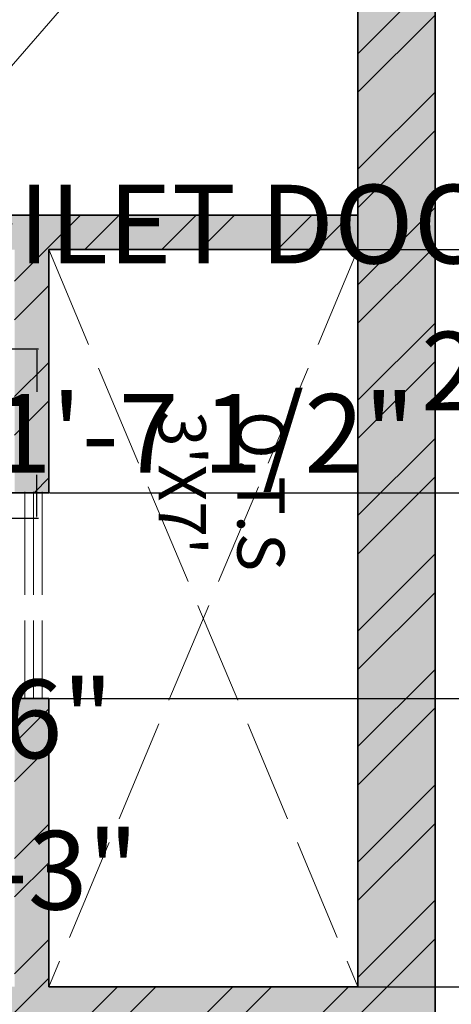
# Model space of a CAD drawing. Units: inches. Extents: x 1086 to 1540, y 3343 to 3848.
# Tile 5 of 8: x 1422 to 1473, y 3547 to 3661. Entities that reach past the tile are written whole.
import ezdxf

# ---------------------------------------------------------------- set-up
doc = ezdxf.new("R2010")
doc.units = ezdxf.units.IN
doc.linetypes.add('ACAD_ISO02W100', pattern=[15, 12, -3])
for name, color, linetype, lineweight in [('00 FURNITURE', 15, 'Continuous', 15), ('A-ANNO-DIMS', 2, 'Continuous', 13), ('A-AREA-IDEN', 7, 'Continuous', 18), ('A-FLOR-OPEN', 8, 'ACAD_ISO02W100', 13), ('A-GLAZ-VENT', 6, 'ACAD_ISO02W100', 13), ('A-WALL-PATT', 252, 'Continuous', 9), ('WALL', 7, 'Continuous', 35)]:
    doc.layers.add(name, color=color, linetype=linetype, lineweight=lineweight)
doc.styles.get("Standard").update_dxf_attribs({"font": 'arial.ttf'})
doc.dimstyles.get("Standard").update_dxf_attribs({"dimtxt": 9.18, "dimasz": 0.18, "dimexe": 0.18, "dimexo": 0.0625, "dimgap": 0.09, "dimtad": 0, "dimtih": 1, "dimtoh": 1, "dimdec": 1, "dimzin": 0, "dimdsep": 46, "dimlunit": 3, "dimtxsty": 'Standard', "dimcen": 0.09, "dimadec": 0, "dimazin": 0, "dimtfac": 1, "dimtdec": 1, "dimtofl": 0, "dimtmove": 0, "dimatfit": 3, "dimfxl": 1, "dimtolj": 1, "dimtzin": 0, "dimarcsym": 0})

# ---------------------------------------------------------------- blocks, each defined once
blk = doc.blocks.new('chair')
at = {"layer": '00 FURNITURE'}
for p, q in [((1375.85, 3529.75), (1402.12, 3529.75)), ((1373.66, 3525.37), (1373.66, 3527.56)), ((1404.31, 3527.56), (1404.31, 3496.9)), ((1371.47, 3525.37), (1397.74, 3525.37)), ((1395.55, 3525.37), (1395.55, 3499.09)), ((1369.28, 3501.28), (1369.28, 3523.18)), ((1399.93, 3523.18), (1399.93, 3501.28)), ((1397.74, 3499.09), (1371.47, 3499.09)), ((1373.66, 3496.9), (1373.66, 3499.09)), ((1402.12, 3494.71), (1375.85, 3494.71))]:
    blk.add_line(p, q, dxfattribs=at)
for centre, start, end in [((1375.85, 3527.56), 90, 180), ((1402.12, 3527.56), 0, 90), ((1371.47, 3523.18), 90, 180), ((1397.74, 3523.18), 0, 90), ((1371.47, 3501.28), 180, 270), ((1397.74, 3501.28), 270, 0), ((1375.85, 3496.9), 180, 270), ((1402.12, 3496.9), 270, 0)]:
    blk.add_arc(centre, 2.19, start, end, dxfattribs=at)
blk = doc.blocks.new('*D13')
at = {"layer": 'A-ANNO-DIMS', "color": 0, "lineweight": -2, "transparency": 16777216}
for p, q in [((1470.8, 3811.57), (1506.93, 3811.57)), ((1506.75, 3811.39), (1506.75, 3600.35)), ((1506.75, 3379.75), (1506.75, 3590.79)), ((1470.8, 3379.57), (1506.93, 3379.57))]:
    blk.add_line(p, q, dxfattribs=at)
at = {"layer": 'A-ANNO-DIMS', "color": 0, "transparency": 16777216}
for points in [[(1506.72, 3811.39), (1506.78, 3811.39), (1506.75, 3811.57)], [(1506.72, 3379.75), (1506.78, 3379.75), (1506.75, 3379.57)]]:
    blk.add_solid(points, dxfattribs=at)
at = {"layer": 'Defpoints', "color": 0, "transparency": 16777216}
for p in [(1470.74, 3811.57), (1470.74, 3379.57), (1506.75, 3379.57)]:
    blk.add_point(p, dxfattribs=at)
at = {"layer": 'A-ANNO-DIMS', "color": 0, "transparency": 16777216, "insert": (1506.75, 3595.57), "char_height": 9.18, "attachment_point": 5}
blk.add_mtext("\\A1;36'", dxfattribs=at)
blk = doc.blocks.new('*D32')
at = {"layer": 'A-ANNO-DIMS', "color": 0, "lineweight": -2, "transparency": 16777216}
for p, q in [((1437.74, 3674.1), (1437.74, 3668.06)), ((1461.74, 3674.1), (1461.74, 3668.06)), ((1437.74, 3668.24), (1437.56, 3668.24)), ((1461.56, 3668.24), (1437.92, 3668.24))]:
    blk.add_line(p, q, dxfattribs=at)
at = {"layer": 'A-ANNO-DIMS', "color": 0, "transparency": 16777216}
for points in [[(1437.92, 3668.27), (1437.92, 3668.21), (1437.74, 3668.24)], [(1461.56, 3668.27), (1461.56, 3668.21), (1461.74, 3668.24)]]:
    blk.add_solid(points, dxfattribs=at)
at = {"layer": 'Defpoints', "color": 0, "transparency": 16777216}
for p in [(1437.74, 3674.16), (1461.74, 3674.16), (1437.74, 3668.24)]:
    blk.add_point(p, dxfattribs=at)
at = {"layer": 'A-ANNO-DIMS', "color": 0, "transparency": 16777216, "insert": (1409.41, 3668.24), "char_height": 9.18, "attachment_point": 5}
blk.add_mtext('\\A1;2\'-0" TYP.', dxfattribs=at)
blk = doc.blocks.new('*D35')
at = {"layer": 'A-ANNO-DIMS', "color": 0, "lineweight": -2, "transparency": 16777216}
for p, q in [((1407.44, 3575.74), (1411.63, 3575.74)), ((1411.45, 3575.56), (1411.45, 3566.99)), ((1411.45, 3548.75), (1411.45, 3557.32)), ((1407.44, 3548.57), (1411.63, 3548.57))]:
    blk.add_line(p, q, dxfattribs=at)
at = {"layer": 'A-ANNO-DIMS', "color": 0, "transparency": 16777216}
for points in [[(1411.42, 3575.56), (1411.48, 3575.56), (1411.45, 3575.74)], [(1411.42, 3548.75), (1411.48, 3548.75), (1411.45, 3548.57)]]:
    blk.add_solid(points, dxfattribs=at)
at = {"layer": 'Defpoints', "color": 0, "transparency": 16777216}
for p in [(1407.37, 3575.74), (1407.37, 3548.57), (1411.45, 3548.57)]:
    blk.add_point(p, dxfattribs=at)
at = {"layer": 'A-ANNO-DIMS', "color": 0, "transparency": 16777216, "insert": (1411.45, 3562.16), "char_height": 9.18, "attachment_point": 5}
blk.add_mtext('\\A1;WC 2\'-3"', dxfattribs=at)
blk = doc.blocks.new('*D36')
at = {"layer": 'A-ANNO-DIMS', "color": 0, "lineweight": -2, "transparency": 16777216}
for p, q in [((1389.26, 3575.8), (1389.26, 3579.99)), ((1389.44, 3579.81), (1407.19, 3579.81)), ((1407.37, 3575.8), (1407.37, 3579.99)), ((1407.37, 3579.81), (1407.55, 3579.81))]:
    blk.add_line(p, q, dxfattribs=at)
at = {"layer": 'A-ANNO-DIMS', "color": 0, "transparency": 16777216}
for points in [[(1389.44, 3579.84), (1389.44, 3579.78), (1389.26, 3579.81)], [(1407.19, 3579.84), (1407.19, 3579.78), (1407.37, 3579.81)]]:
    blk.add_solid(points, dxfattribs=at)
at = {"layer": 'Defpoints', "color": 0, "transparency": 16777216}
for p in [(1407.37, 3579.81), (1389.26, 3575.74), (1407.37, 3575.74)]:
    blk.add_point(p, dxfattribs=at)
at = {"layer": 'A-ANNO-DIMS', "color": 0, "transparency": 16777216, "insert": (1419.41, 3579.81), "char_height": 9.18, "attachment_point": 5}
blk.add_mtext('\\A1;1\'-6"', dxfattribs=at)
blk = doc.blocks.new('*D37')
at = {"layer": 'A-ANNO-DIMS', "color": 0, "lineweight": -2, "transparency": 16777216}
for p, q in [((1421.44, 3623), (1424.52, 3623)), ((1424.34, 3622.82), (1424.34, 3617.96)), ((1424.34, 3603.43), (1424.34, 3608.29)), ((1421.44, 3603.25), (1424.52, 3603.25))]:
    blk.add_line(p, q, dxfattribs=at)
at = {"layer": 'A-ANNO-DIMS', "color": 0, "transparency": 16777216}
for points in [[(1424.31, 3622.82), (1424.37, 3622.82), (1424.34, 3623)], [(1424.31, 3603.43), (1424.37, 3603.43), (1424.34, 3603.25)]]:
    blk.add_solid(points, dxfattribs=at)
at = {"layer": 'Defpoints', "color": 0, "transparency": 16777216}
for p in [(1421.38, 3623), (1424.34, 3623), (1421.38, 3603.25)]:
    blk.add_point(p, dxfattribs=at)
at = {"layer": 'A-ANNO-DIMS', "color": 0, "transparency": 16777216, "insert": (1424.34, 3613.12), "char_height": 9.18, "attachment_point": 5}
blk.add_mtext('\\A1;BASIN 1\'-7 1/2"', dxfattribs=at)
blk = doc.blocks.new('*D41')
at = {"layer": 'A-ANNO-DIMS', "color": 0, "lineweight": -2, "transparency": 16777216}
for p, q in [((1369.71, 3632.63), (1369.71, 3637.72)), ((1369.89, 3637.54), (1402.67, 3637.54)), ((1402.85, 3632.63), (1402.85, 3637.72)), ((1402.85, 3637.54), (1403.03, 3637.54))]:
    blk.add_line(p, q, dxfattribs=at)
at = {"layer": 'A-ANNO-DIMS', "color": 0, "transparency": 16777216}
for points in [[(1369.89, 3637.57), (1369.89, 3637.51), (1369.71, 3637.54)], [(1402.67, 3637.57), (1402.67, 3637.51), (1402.85, 3637.54)]]:
    blk.add_solid(points, dxfattribs=at)
at = {"layer": 'Defpoints', "color": 0, "transparency": 16777216}
for p in [(1402.85, 3637.54), (1369.71, 3632.57), (1402.85, 3632.57)]:
    blk.add_point(p, dxfattribs=at)
at = {"layer": 'A-ANNO-DIMS', "color": 0, "transparency": 16777216, "insert": (1460.68, 3637.54), "char_height": 9.18, "attachment_point": 5}
blk.add_mtext('\\A1;TOILET DOOR 2\'-9"', dxfattribs=at)
blk = doc.blocks.new('*D67')
at = {"layer": 'A-ANNO-DIMS', "color": 0, "lineweight": -2, "transparency": 16777216}
for p, q in [((1425.8, 3606.21), (1493.92, 3606.21)), ((1493.74, 3606.03), (1493.74, 3598.99)), ((1493.74, 3582.39), (1493.74, 3589.44)), ((1425.8, 3582.21), (1493.92, 3582.21))]:
    blk.add_line(p, q, dxfattribs=at)
at = {"layer": 'A-ANNO-DIMS', "color": 0, "transparency": 16777216}
for points in [[(1493.71, 3606.03), (1493.77, 3606.03), (1493.74, 3606.21)], [(1493.71, 3582.39), (1493.77, 3582.39), (1493.74, 3582.21)]]:
    blk.add_solid(points, dxfattribs=at)
at = {"layer": 'Defpoints', "color": 0, "transparency": 16777216}
for p in [(1425.74, 3606.21), (1493.74, 3606.21), (1425.74, 3582.21)]:
    blk.add_point(p, dxfattribs=at)
at = {"layer": 'A-ANNO-DIMS', "color": 0, "transparency": 16777216, "insert": (1493.74, 3594.21), "char_height": 9.18, "attachment_point": 5}
blk.add_mtext('\\A1;2\'-0"', dxfattribs=at)
blk = doc.blocks.new('*D68')
at = {"layer": 'A-ANNO-DIMS', "color": 0, "lineweight": -2, "transparency": 16777216}
for p, q in [((1425.8, 3634.57), (1493.92, 3634.57)), ((1493.74, 3634.39), (1493.74, 3625.23)), ((1493.74, 3606.39), (1493.74, 3615.56)), ((1425.8, 3606.21), (1493.92, 3606.21))]:
    blk.add_line(p, q, dxfattribs=at)
at = {"layer": 'A-ANNO-DIMS', "color": 0, "transparency": 16777216}
for points in [[(1493.71, 3634.39), (1493.77, 3634.39), (1493.74, 3634.57)], [(1493.71, 3606.39), (1493.77, 3606.39), (1493.74, 3606.21)]]:
    blk.add_solid(points, dxfattribs=at)
at = {"layer": 'Defpoints', "color": 0, "transparency": 16777216}
for p in [(1425.74, 3634.57), (1493.74, 3634.57), (1425.74, 3606.21)]:
    blk.add_point(p, dxfattribs=at)
at = {"layer": 'A-ANNO-DIMS', "color": 0, "transparency": 16777216, "insert": (1493.74, 3620.39), "char_height": 9.18, "attachment_point": 5}
blk.add_mtext('\\A1;2\'-4 1/2"', dxfattribs=at)
blk = doc.blocks.new('*D71')
at = {"layer": 'A-ANNO-DIMS', "color": 0, "lineweight": -2, "transparency": 16777216}
for p, q in [((1461.8, 3634.57), (1493.92, 3634.57)), ((1493.74, 3634.39), (1493.74, 3596.27)), ((1493.74, 3548.75), (1493.74, 3586.87)), ((1461.8, 3548.57), (1493.92, 3548.57))]:
    blk.add_line(p, q, dxfattribs=at)
at = {"layer": 'A-ANNO-DIMS', "color": 0, "transparency": 16777216}
for points in [[(1493.71, 3634.39), (1493.77, 3634.39), (1493.74, 3634.57)], [(1493.71, 3548.75), (1493.77, 3548.75), (1493.74, 3548.57)]]:
    blk.add_solid(points, dxfattribs=at)
at = {"layer": 'Defpoints', "color": 0, "transparency": 16777216}
for p in [(1461.74, 3634.57), (1493.74, 3634.57), (1461.74, 3548.57)]:
    blk.add_point(p, dxfattribs=at)
at = {"layer": 'A-ANNO-DIMS', "color": 0, "transparency": 16777216, "insert": (1493.74, 3591.57), "char_height": 9.18, "attachment_point": 5}
blk.add_mtext('\\A1;7\'-2"', dxfattribs=at)

msp = doc.modelspace()

# ---------------------------------------------------------------- hatches: boundary and pattern name
at = {"layer": 'A-WALL-PATT'}
h = msp.add_hatch(dxfattribs=at)
h.set_pattern_fill('ANSI32', color=256)
h.paths.add_polyline_path([(1234.55, 3811.57), (1234.55, 3811.57), (1194.74, 3811.57), (1194.74, 3622.57), (1203.74, 3622.57), (1203.74, 3634.57), (1218.33, 3634.57), (1218.33, 3638.57), (1203.74, 3638.57), (1203.74, 3802.57), (1234.55, 3802.57)])
h.paths.add_polyline_path([(1371.06, 3811.57), (1371.06, 3811.57), (1282.55, 3811.57), (1282.55, 3802.57), (1331.74, 3802.57), (1331.74, 3634.57), (1335.74, 3634.57), (1335.74, 3639.57), (1335.74, 3802.57), (1371.06, 3802.57)])
h.paths.add_polyline_path([(1470.74, 3811.57), (1419.06, 3811.57), (1419.06, 3802.57), (1461.74, 3802.57), (1461.74, 3638.57), (1461.74, 3548.57), (1425.74, 3548.57), (1425.74, 3582.21), (1421.74, 3582.21), (1421.74, 3548.57), (1376.74, 3548.57), (1376.74, 3602.57), (1373.71, 3602.57), (1372.74, 3602.57), (1372.74, 3544.57), (1461.74, 3544.57), (1461.74, 3379.57), (1470.74, 3379.57)])
h.paths.add_polyline_path([(1203.74, 3582.57), (1295.74, 3582.57), (1295.74, 3586.57), (1203.74, 3586.57), (1203.74, 3598.57), (1194.74, 3598.57), (1194.74, 3379.57), (1326.74, 3379.57), (1326.74, 3388.57), (1322.74, 3388.57), (1203.74, 3388.57), (1203.74, 3451.57), (1234.74, 3451.57), (1234.74, 3455.57), (1203.74, 3455.57), (1203.74, 3479.57), (1203.74, 3544.57), (1227.74, 3544.57), (1253.74, 3544.57), (1253.74, 3548.57), (1203.74, 3548.57)])
h.paths.add_polyline_path([(1461.74, 3638.57), (1371.74, 3638.57), (1371.74, 3634.57), (1372.74, 3634.57), (1372.74, 3632.57), (1376.74, 3632.57), (1376.74, 3634.57), (1421.74, 3634.57), (1421.74, 3606.21), (1425.74, 3606.21), (1425.74, 3634.57), (1461.74, 3634.57)])
h.paths.add_polyline_path([(1295.74, 3638.57), (1266.33, 3638.57), (1266.33, 3634.57), (1292.74, 3634.57), (1295.74, 3634.57)])
h.paths.add_polyline_path([(1322.74, 3548.57), (1318.74, 3548.57), (1318.74, 3455.57), (1282.74, 3455.57), (1282.74, 3451.57), (1318.74, 3451.57), (1318.74, 3420.07), (1322.74, 3420.07)], flags=17)
at = {"layer": 'A-WALL-PATT', "transparency": 33554559}
h = msp.add_hatch(color=256, dxfattribs=at)
h.dxf.hatch_style = 1
h.paths.add_polyline_path([(1234.55, 3811.57), (1234.55, 3811.57), (1194.74, 3811.57), (1194.74, 3622.57), (1203.74, 3622.57), (1203.74, 3634.57), (1218.33, 3634.57), (1218.33, 3638.57), (1203.74, 3638.57), (1203.74, 3802.57), (1234.55, 3802.57)])
h.paths.add_polyline_path([(1371.06, 3811.57), (1371.06, 3811.57), (1282.55, 3811.57), (1282.55, 3802.57), (1331.74, 3802.57), (1331.74, 3634.57), (1335.74, 3634.57), (1335.74, 3639.57), (1335.74, 3802.57), (1371.06, 3802.57)])
h.paths.add_polyline_path([(1470.74, 3811.57), (1419.06, 3811.57), (1419.06, 3802.57), (1461.74, 3802.57), (1461.74, 3638.57), (1461.74, 3548.57), (1425.74, 3548.57), (1425.74, 3582.21), (1421.74, 3582.21), (1421.74, 3548.57), (1376.74, 3548.57), (1376.74, 3602.57), (1372.74, 3602.57), (1372.74, 3544.57), (1461.74, 3544.57), (1461.74, 3379.57), (1470.74, 3379.57)])
h.paths.add_polyline_path([(1203.74, 3544.57), (1227.74, 3544.57), (1253.74, 3544.57), (1253.74, 3548.57), (1203.74, 3548.57), (1203.74, 3582.57), (1295.74, 3582.57), (1295.74, 3586.57), (1203.74, 3586.57), (1203.74, 3598.57), (1194.74, 3598.57), (1194.74, 3379.57), (1326.74, 3379.57), (1326.74, 3388.57), (1322.74, 3388.57), (1203.74, 3388.57), (1203.74, 3451.57), (1234.74, 3451.57), (1234.74, 3455.57), (1203.74, 3455.57)])
h.paths.add_polyline_path([(1413.74, 3388.57), (1413.74, 3388.57), (1374.74, 3388.57), (1374.74, 3383.18), (1374.74, 3383.18), (1374.74, 3379.57), (1413.74, 3379.57)], flags=17)
h.paths.add_polyline_path([(1322.74, 3548.57), (1318.74, 3548.57), (1318.74, 3455.57), (1282.74, 3455.57), (1282.74, 3451.57), (1318.74, 3451.57), (1318.74, 3420.07), (1322.74, 3420.07)], flags=17)
h.paths.add_polyline_path([(1295.74, 3638.57), (1266.33, 3638.57), (1266.33, 3634.57), (1292.74, 3634.57), (1295.74, 3634.57)])
h.paths.add_polyline_path([(1461.74, 3638.57), (1371.74, 3638.57), (1371.74, 3634.57), (1372.74, 3634.57), (1372.74, 3632.57), (1376.74, 3632.57), (1376.74, 3634.57), (1421.74, 3634.57), (1421.74, 3606.21), (1425.74, 3606.21), (1425.74, 3634.57), (1461.74, 3634.57)])

# ---------------------------------------------------------------- linework, layer by layer
at = {"layer": 'A-FLOR-OPEN'}
for p, q in [((1425.74, 3634.57), (1461.74, 3548.57)), ((1461.74, 3634.57), (1425.74, 3548.57))]:
    msp.add_line(p, q, dxfattribs=at)
at = {"layer": 'A-GLAZ-VENT'}
for p, q in [((1422.94, 3606.31), (1422.94, 3582.31)), ((1423.94, 3606.31), (1423.94, 3582.31)), ((1424.94, 3606.31), (1424.94, 3582.31))]:
    msp.add_line(p, q, dxfattribs=at)
at = {"layer": 'WALL'}
for p, q in [((1470.74, 3811.57), (1470.74, 3379.57)), ((1461.74, 3802.57), (1461.74, 3638.57)), ((1371.74, 3638.57), (1461.74, 3638.57)), ((1461.74, 3638.57), (1461.74, 3548.57)), ((1425.74, 3634.57), (1425.74, 3606.21)), ((1425.74, 3634.57), (1461.74, 3634.57)), ((1425.74, 3606.21), (1421.38, 3606.21)), ((1425.74, 3582.21), (1421.74, 3582.21)), ((1425.74, 3582.21), (1425.74, 3548.57)), ((1425.74, 3548.57), (1461.74, 3548.57))]:
    msp.add_line(p, q, dxfattribs=at)

# ---------------------------------------------------------------- block references
at = {"layer": '00 FURNITURE', "xscale": -1, "rotation": 228.9612801357977}
msp.add_blockref('chair', (-2148.96, 4930.45), dxfattribs=at)

# ---------------------------------------------------------------- texts
at = {"layer": 'A-AREA-IDEN', "insert": (1453.2, 3615.75), "char_height": 8, "attachment_point": 1, "rotation": 270}
msp.add_mtext_dynamic_manual_height_columns("{\\H0.6875x;O.T.S\\P3'X7'}  ", width=58.9878, gutter_width=0, heights=[37.04], dxfattribs=at)

# ---------------------------------------------------------------- dimensions: what is measured, and where the dimension line sits
at = {"layer": 'A-ANNO-DIMS'}
for base, p1, p2, override, picture, middle in [((1506.75, 3379.57), (1470.74, 3811.57), (1470.74, 3379.57), {"dimclrd": 0, "dimclre": 0, "dimclrt": 0}, '*D13', (1506.75, 3595.57)), ((1493.74, 3634.57), (1425.74, 3606.21), (1425.74, 3634.57), {"dimdec": 1, "dimlfac": 1, "dimrnd": 0, "dimzin": 1, "dimdsep": 46, "dimlunit": 4, "dimfrac": 2}, '*D68', (1493.74, 3620.39)), ((1493.74, 3634.57), (1461.74, 3548.57), (1461.74, 3634.57), {"dimdec": 1, "dimlfac": 1, "dimrnd": 0, "dimzin": 1, "dimdsep": 46, "dimlunit": 4, "dimfrac": 2}, '*D71', (1493.74, 3591.57)), ((1493.74, 3606.21), (1425.74, 3582.21), (1425.74, 3606.21), {"dimdec": 1, "dimlfac": 1, "dimrnd": 0, "dimzin": 1, "dimdsep": 46, "dimlunit": 4, "dimfrac": 2}, '*D67', (1493.74, 3594.21))]:
    dim = msp.add_linear_dim(base=base, p1=p1, p2=p2, angle=90, dimstyle='Standard', override=override, dxfattribs=at)
    dim.commit()
    dim.dimension.update_dxf_attribs({"geometry": picture, "text_midpoint": middle})
for base, p1, p2, angle, text, picture, middle in [((1437.74, 3668.24), (1461.74, 3674.16), (1437.74, 3674.16), 180, '<> TYP.', '*D32', (1409.41, 3668.24)), ((1424.3405, 3622.9968), (1421.3787, 3603.2512), (1421.3787, 3622.9968), 90, 'BASIN <>', '*D37', (1424.3405, 3613.124)), ((1411.45, 3548.57), (1407.37, 3575.74), (1407.37, 3548.57), 270, 'WC <>', '*D35', (1411.45, 3562.16))]:
    dim = msp.add_linear_dim(base=base, p1=p1, p2=p2, angle=angle, text=text, dimstyle='Standard', override={"dimdec": 1, "dimlfac": 1, "dimrnd": 0, "dimzin": 1, "dimdsep": 46, "dimlunit": 4, "dimfrac": 2}, dxfattribs=at)
    dim.commit()
    dim.dimension.update_dxf_attribs({"geometry": picture, "text_midpoint": middle})
dim = msp.add_linear_dim(base=(1402.85, 3637.54), p1=(1369.71, 3632.57), p2=(1402.85, 3632.57), text='TOILET DOOR <>', dimstyle='Standard', override={"dimdec": 1, "dimlfac": 1, "dimrnd": 0, "dimzin": 1, "dimdsep": 46, "dimlunit": 4, "dimfrac": 2}, dxfattribs=at)
dim.commit()
dim.dimension.update_dxf_attribs({"geometry": '*D41', "text_midpoint": (1460.68, 3637.54)})
dim = msp.add_linear_dim(base=(1407.37, 3579.81), p1=(1389.26, 3575.74), p2=(1407.37, 3575.74), dimstyle='Standard', override={"dimdec": 1, "dimlfac": 1, "dimrnd": 0, "dimzin": 1, "dimdsep": 46, "dimlunit": 4, "dimfrac": 2}, dxfattribs=at)
dim.commit()
dim.dimension.update_dxf_attribs({"geometry": '*D36', "text_midpoint": (1419.41, 3579.81)})

doc.saveas('drawing.dxf')
